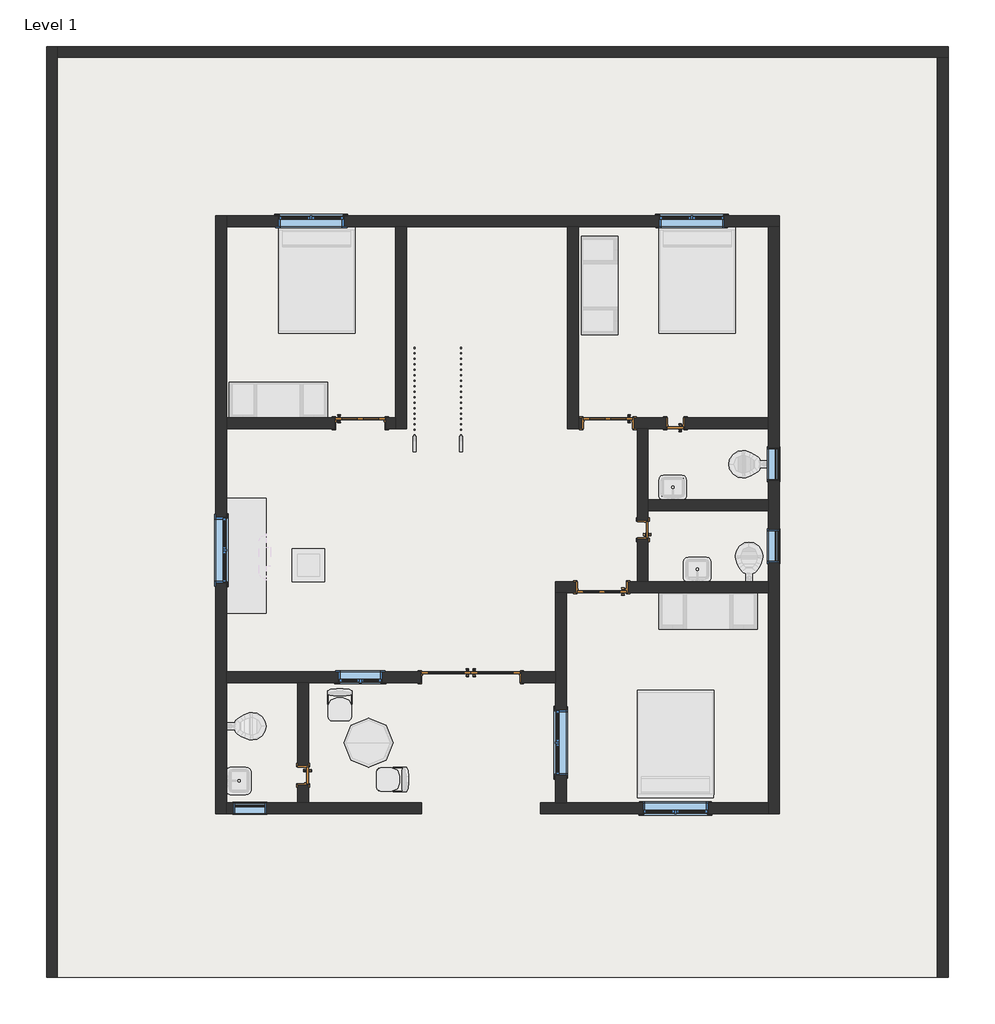
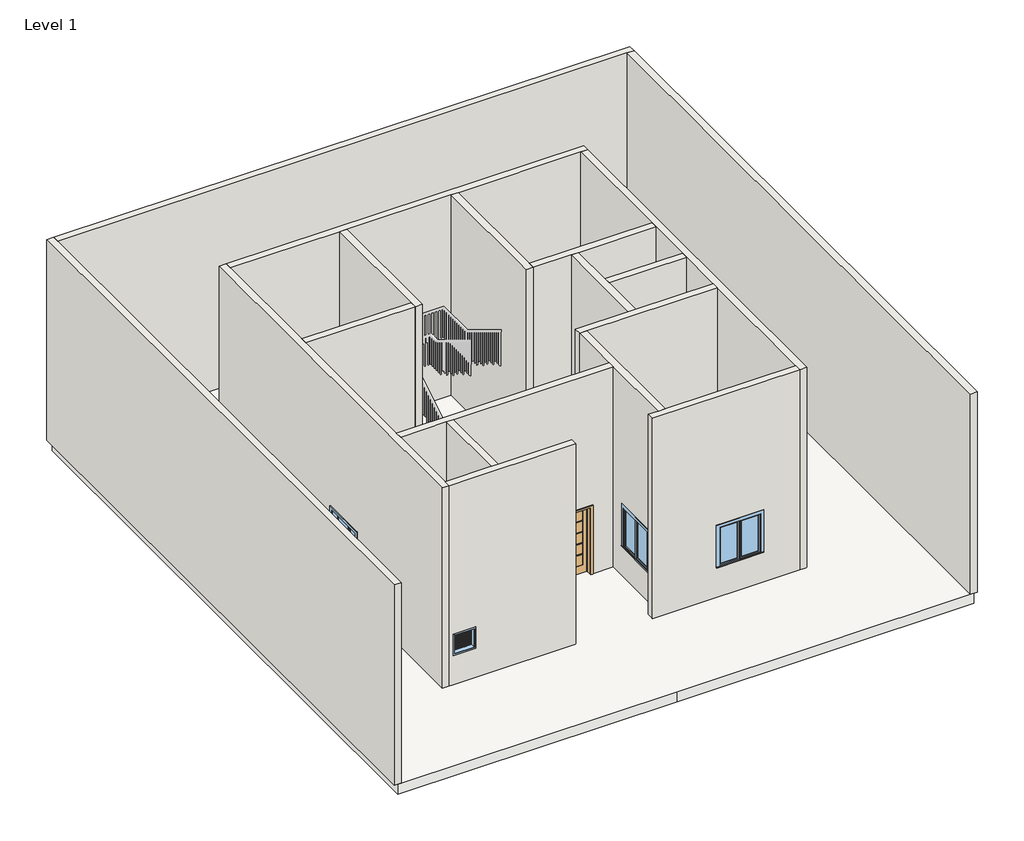
# One storey, part 1 of 3: 18 walls, 9 windows, 7 doors, 1 slab.
"""IFC4 building model written with IfcOpenShell, lengths in millimetres."""

from ifc_helpers import new_model, si_unit, frame, origin, origin_with_axes, place, context, project, spatial, polyline, outline, extrude, faceted_brep, transform, mapped, element, save
from components import door_48c357d2, door_5dfbd760, door_c2afa946, door_21b72c96, door_b2d2822a, window_bb17773d, window_0862ab64, window_0038ecf3, window_75debfae

model = new_model("IFC4")

# Units and contexts
model_context = context("Model", 3, world=origin())
ifc_project = project(units=[si_unit("LENGTHUNIT", "METRE", prefix="MILLI")], contexts=[model_context])

# Site, building, storey
site = spatial("IfcSite", under=ifc_project)
building = spatial("IfcBuilding", under=site)
storey = spatial("IfcBuildingStorey", under=building, Name="Level 1", Elevation=0.0)

# Doors
placement = place(None, origin())
door_shape = door_48c357d2(model_context)
element("IfcDoor", 1, ObjectType="Door-Interior-Double-Full Glass-Wood : 72\" x 80\"", at=placement, inside=storey, context=model_context, shape_type="MappedRepresentation", body=[
    mapped(door_shape, transform((-7146.8868169, 4286.8240268, 0.0), x_axis=(1.0, 0.0, 0.0), y_axis=(0.0, 1.0, 0.0), z_axis=(0.0, 0.0, 1.0))),
])
door_2_shape = door_5dfbd760(model_context)
element("IfcDoor", 2, ObjectType="Door-Interior-Single-6_Panel-Wood : 36\" x 80\"", at=placement, inside=storey, context=model_context, shape_type="MappedRepresentation", body=[
    mapped(door_2_shape, transform((-9204.2868169, 9011.2240268, 0.0), x_axis=(1.0, 0.0, 0.0), y_axis=(0.0, 1.0, 0.0), z_axis=(0.0, 0.0, 1.0))),
])
element("IfcDoor", 3, ObjectType="Door-Interior-Single-6_Panel-Wood : 36\" x 80\"", at=placement, inside=storey, context=model_context, shape_type="MappedRepresentation", body=[
    mapped(door_2_shape, transform((-4708.4868169, 5956.8740268, 0.0), x_axis=(-1.0, 0.0, 0.0), y_axis=(0.0, -1.0, 0.0), z_axis=(0.0, 0.0, 1.0))),
])
door_3_shape = door_c2afa946(model_context)
element("IfcDoor", 4, ObjectType="Door-Interior-Single-6_Panel-Wood : 36\" x 80\"", at=placement, inside=storey, context=model_context, shape_type="MappedRepresentation", body=[
    mapped(door_3_shape, transform((-4594.1868169, 9011.2240268, 0.0), x_axis=(-1.0, 0.0, 0.0), y_axis=(0.0, -1.0, 0.0), z_axis=(0.0, 0.0, 1.0))),
])
door_4_shape = door_21b72c96(model_context)
element("IfcDoor", 5, ObjectType="Door-Interior-Single-Flush_Panel-Wood : 12\" x 80\"", at=placement, inside=storey, context=model_context, shape_type="MappedRepresentation", body=[
    mapped(door_4_shape, transform((-3943.3118169, 7026.8490268, 0.0), x_axis=(0.0, 1.0, 0.0), y_axis=(-1.0, 0.0, 0.0), z_axis=(0.0, 0.0, 1.0))),
])
door_5_shape = door_b2d2822a(model_context)
element("IfcDoor", 6, ObjectType="Door-Interior-Single-Flush_Panel-Wood : 12\" x 80\"", at=placement, inside=storey, context=model_context, shape_type="MappedRepresentation", body=[
    mapped(door_5_shape, transform((-3336.8868169, 9004.8740268, 0.0), x_axis=(-1.0, 0.0, 0.0), y_axis=(0.0, -1.0, 0.0), z_axis=(0.0, 0.0, 1.0))),
])
element("IfcDoor", 7, ObjectType="Door-Interior-Single-Flush_Panel-Wood : 12\" x 80\"", at=placement, inside=storey, context=model_context, shape_type="MappedRepresentation", body=[
    mapped(door_5_shape, transform((-10267.9118169, 2454.8490268, 0.0), x_axis=(0.0, -1.0, 0.0), y_axis=(1.0, 0.0, 0.0), z_axis=(0.0, 0.0, 1.0))),
])

# Slab
element("IfcSlab", 8, ObjectType="Generic - 12\"", at=placement, inside=storey, context=model_context, shape_type="SweptSolid", body=[
    extrude(outline(polyline([(-14944.6868169, 15916.8490268), (1641.5131831, 15916.8490268), (1641.5131831, -1304.3509732), (-6893.7351469, -1304.3509732), (-14944.6868169, -1304.3509732), (-14944.6868169, 15916.8490268)])), frame((0.0, 0.0, -304.8), z_axis=(0.0, 0.0, 1.0), x_axis=(1.0, 0.0, 0.0)), (0.0, 0.0, 1.0), 304.8),
])

# Walls
element("IfcWall", 9, ObjectType="Generic - 8\"", at=placement, inside=storey, context=model_context, shape_type="Brep", body=[
    faceted_brep([(-11693.4868169, 12665.6490268, 0.0), (-8543.8868169, 12665.6490268, 0.0), (-8340.6868169, 12665.6490268, 0.0), (-5343.4868169, 12665.6490268, 0.0), (-5140.2868169, 12665.6490268, 0.0), (-1609.6868169, 12665.6490268, 0.0), (-1406.4868169, 12665.6490268, 0.0), (-1406.4868169, 12665.6490268, 6096.0), (-1609.6868169, 12665.6490268, 6096.0), (-5140.2868169, 12665.6490268, 6096.0), (-5343.4868169, 12665.6490268, 6096.0), (-8340.6868169, 12665.6490268, 6096.0), (-8543.8868169, 12665.6490268, 6096.0), (-11693.4868169, 12665.6490268, 6096.0), (-2422.4868169, 12665.6490268, 2133.6), (-2422.4868169, 12665.6490268, 914.4), (-3641.6868169, 12665.6490268, 914.4), (-3641.6868169, 12665.6490268, 2133.6), (-9509.0868169, 12665.6490268, 2133.6), (-9509.0868169, 12665.6490268, 914.4), (-10728.2868169, 12665.6490268, 914.4), (-10728.2868169, 12665.6490268, 2133.6), (-11693.4868169, 12868.8490268, 0.0), (-11693.4868169, 12868.8490268, 6096.0), (-1406.4868169, 12868.8490268, 6096.0), (-1406.4868169, 12868.8490268, 0.0), (-2422.4868169, 12868.8490268, 2133.6), (-3641.6868169, 12868.8490268, 2133.6), (-3641.6868169, 12868.8490268, 914.4), (-2422.4868169, 12868.8490268, 914.4), (-9509.0868169, 12868.8490268, 2133.6), (-10728.2868169, 12868.8490268, 2133.6), (-10728.2868169, 12868.8490268, 914.4), (-9509.0868169, 12868.8490268, 914.4)], [[[0, 1, 2, 3, 4, 5, 6, 7, 8, 9, 10, 11, 12, 13], [14, 15, 16, 17], [18, 19, 20, 21]], [[22, 23, 24, 25], [26, 27, 28, 29], [30, 31, 32, 33]], [[6, 5, 4, 3, 2, 1, 0, 22, 25]], [[13, 12, 11, 10, 9, 8, 7, 24, 23]], [[7, 6, 25, 24]], [[0, 13, 23, 22]], [[15, 14, 26, 29]], [[16, 15, 29, 28]], [[17, 16, 28, 27]], [[14, 17, 27, 26]], [[19, 18, 30, 33]], [[20, 19, 33, 32]], [[21, 20, 32, 31]], [[18, 21, 31, 30]]]),
])
element("IfcWall", 10, ObjectType="Generic - 8\"", at=placement, inside=storey, context=model_context, shape_type="Brep", body=[
    faceted_brep([(-1609.6868169, 12665.6490268, 0.0), (-1609.6868169, 9109.6490268, 0.0), (-1609.6868169, 8906.4490268, 0.0), (-1609.6868169, 7585.6490268, 0.0), (-1609.6868169, 7382.4490268, 0.0), (-1609.6868169, 6061.6490268, 0.0), (-1609.6868169, 5858.4490268, 0.0), (-1609.6868169, 1946.8490268, 0.0), (-1609.6868169, 1743.6490268, 0.0), (-1609.6868169, 1743.6490268, 6096.0), (-1609.6868169, 1946.8490268, 6096.0), (-1609.6868169, 5858.4490268, 6096.0), (-1609.6868169, 6061.6490268, 6096.0), (-1609.6868169, 7382.4490268, 6096.0), (-1609.6868169, 7585.6490268, 6096.0), (-1609.6868169, 8906.4490268, 6096.0), (-1609.6868169, 9109.6490268, 6096.0), (-1609.6868169, 12665.6490268, 6096.0), (-1609.6868169, 6417.2490268, 1524.0), (-1609.6868169, 6417.2490268, 914.4), (-1609.6868169, 7026.8490268, 914.4), (-1609.6868169, 7026.8490268, 1524.0), (-1609.6868169, 7941.2490268, 1524.0), (-1609.6868169, 7941.2490268, 914.4), (-1609.6868169, 8550.8490268, 914.4), (-1609.6868169, 8550.8490268, 1524.0), (-1406.4868169, 12665.6490268, 0.0), (-1406.4868169, 12665.6490268, 6096.0), (-1406.4868169, 1743.6490268, 6096.0), (-1406.4868169, 1743.6490268, 0.0), (-1406.4868169, 6417.2490268, 1524.0), (-1406.4868169, 7026.8490268, 1524.0), (-1406.4868169, 7026.8490268, 914.4), (-1406.4868169, 6417.2490268, 914.4), (-1406.4868169, 7941.2490268, 1524.0), (-1406.4868169, 8550.8490268, 1524.0), (-1406.4868169, 8550.8490268, 914.4), (-1406.4868169, 7941.2490268, 914.4)], [[[0, 1, 2, 3, 4, 5, 6, 7, 8, 9, 10, 11, 12, 13, 14, 15, 16, 17], [18, 19, 20, 21], [22, 23, 24, 25]], [[26, 27, 28, 29], [30, 31, 32, 33], [34, 35, 36, 37]], [[8, 7, 6, 5, 4, 3, 2, 1, 0, 26, 29]], [[17, 16, 15, 14, 13, 12, 11, 10, 9, 28, 27]], [[0, 17, 27, 26]], [[9, 8, 29, 28]], [[19, 18, 30, 33]], [[20, 19, 33, 32]], [[21, 20, 32, 31]], [[18, 21, 31, 30]], [[23, 22, 34, 37]], [[24, 23, 37, 36]], [[25, 24, 36, 35]], [[22, 25, 35, 34]]]),
])
element("IfcWall", 11, ObjectType="Generic - 8\"", at=placement, inside=storey, context=model_context, shape_type="Brep", body=[
    faceted_brep([(-1609.6868169, 1946.8490268, 0.0), (-5368.8868169, 1946.8490268, 0.0), (-5572.0868169, 1946.8490268, 0.0), (-5851.4868169, 1946.8490268, 0.0), (-5851.4868169, 1946.8490268, 6096.0), (-5572.0868169, 1946.8490268, 6096.0), (-5368.8868169, 1946.8490268, 6096.0), (-1609.6868169, 1946.8490268, 6096.0), (-3946.4868169, 1946.8490268, 2133.6), (-3946.4868169, 1946.8490268, 914.4), (-2727.2868169, 1946.8490268, 914.4), (-2727.2868169, 1946.8490268, 2133.6), (-1609.6868169, 1743.6490268, 0.0), (-1609.6868169, 1743.6490268, 6096.0), (-5851.4868169, 1743.6490268, 6096.0), (-5851.4868169, 1743.6490268, 0.0), (-3946.4868169, 1743.6490268, 2133.6), (-2727.2868169, 1743.6490268, 2133.6), (-2727.2868169, 1743.6490268, 914.4), (-3946.4868169, 1743.6490268, 914.4)], [[[0, 1, 2, 3, 4, 5, 6, 7], [8, 9, 10, 11]], [[12, 13, 14, 15], [16, 17, 18, 19]], [[3, 2, 1, 0, 12, 15]], [[4, 3, 15, 14]], [[7, 6, 5, 4, 14, 13]], [[0, 7, 13, 12]], [[9, 8, 16, 19]], [[10, 9, 19, 18]], [[11, 10, 18, 17]], [[8, 11, 17, 16]]]),
])
element("IfcWall", 12, ObjectType="Generic - 8\"", at=placement, inside=storey, context=model_context, shape_type="Brep", body=[
    faceted_brep([(-11693.4868169, 1743.6490268, 0.0), (-11693.4868169, 1946.8490268, 0.0), (-11693.4868169, 4182.0490268, 0.0), (-11693.4868169, 4385.2490268, 0.0), (-11693.4868169, 8906.4490268, 0.0), (-11693.4868169, 9109.6490268, 0.0), (-11693.4868169, 12665.6490268, 0.0), (-11693.4868169, 12868.8490268, 0.0), (-11693.4868169, 12868.8490268, 6096.0), (-11693.4868169, 12665.6490268, 6096.0), (-11693.4868169, 9109.6490268, 6096.0), (-11693.4868169, 8906.4490268, 6096.0), (-11693.4868169, 4385.2490268, 6096.0), (-11693.4868169, 4182.0490268, 6096.0), (-11693.4868169, 1946.8490268, 6096.0), (-11693.4868169, 1743.6490268, 6096.0), (-11693.4868169, 6036.2490268, 2133.6), (-11693.4868169, 7255.4490268, 2133.6), (-11693.4868169, 7255.4490268, 914.4), (-11693.4868169, 6036.2490268, 914.4), (-11896.6868169, 1743.6490268, 0.0), (-11896.6868169, 1743.6490268, 6096.0), (-11896.6868169, 12868.8490268, 6096.0), (-11896.6868169, 12868.8490268, 0.0), (-11896.6868169, 6036.2490268, 2133.6), (-11896.6868169, 6036.2490268, 914.4), (-11896.6868169, 7255.4490268, 914.4), (-11896.6868169, 7255.4490268, 2133.6)], [[[0, 1, 2, 3, 4, 5, 6, 7, 8, 9, 10, 11, 12, 13, 14, 15], [16, 17, 18, 19]], [[20, 21, 22, 23], [24, 25, 26, 27]], [[7, 6, 5, 4, 3, 2, 1, 0, 20, 23]], [[15, 14, 13, 12, 11, 10, 9, 8, 22, 21]], [[8, 7, 23, 22]], [[0, 15, 21, 20]], [[25, 24, 16, 19]], [[26, 25, 19, 18]], [[27, 26, 18, 17]], [[24, 27, 17, 16]]]),
])
element("IfcWall", 13, ObjectType="Generic - 8\"", at=placement, inside=storey, context=model_context, shape_type="Brep", body=[
    faceted_brep([(-8340.6868169, 8906.4490268, 0.0), (-8340.6868169, 12665.6490268, 0.0), (-8340.6868169, 12665.6490268, 6096.0), (-8340.6868169, 8906.4490268, 6096.0), (-8543.8868169, 8906.4490268, 0.0), (-8543.8868169, 8906.4490268, 6096.0), (-8543.8868169, 9109.6490268, 6096.0), (-8543.8868169, 12665.6490268, 6096.0), (-8543.8868169, 12665.6490268, 0.0), (-8543.8868169, 9109.6490268, 0.0)], [[[0, 1, 2, 3]], [[4, 5, 6, 7, 8, 9]], [[1, 0, 4, 9, 8]], [[3, 2, 7, 6, 5]], [[2, 1, 8, 7]], [[0, 3, 5, 4]]]),
])
element("IfcWall", 14, ObjectType="Generic - 8\"", at=placement, inside=storey, context=model_context, shape_type="Brep", body=[
    faceted_brep([(-5140.2868169, 8906.4490268, 0.0), (-5140.2868169, 9109.6490268, 0.0), (-5140.2868169, 12665.6490268, 0.0), (-5140.2868169, 12665.6490268, 6096.0), (-5140.2868169, 9109.6490268, 6096.0), (-5140.2868169, 8906.4490268, 6096.0), (-5343.4868169, 8906.4490268, 0.0), (-5343.4868169, 8906.4490268, 6096.0), (-5343.4868169, 12665.6490268, 6096.0), (-5343.4868169, 12665.6490268, 0.0)], [[[0, 1, 2, 3, 4, 5]], [[6, 7, 8, 9]], [[2, 1, 0, 6, 9]], [[5, 4, 3, 8, 7]], [[3, 2, 9, 8]], [[0, 5, 7, 6]]]),
])
element("IfcWall", 15, ObjectType="Generic - 8\"", at=placement, inside=storey, context=model_context, shape_type="Brep", body=[
    faceted_brep([(-1609.6868169, 8906.4490268, 6096.0), (-3844.8868169, 8906.4490268, 6096.0), (-4048.0868169, 8906.4490268, 6096.0), (-5140.2868169, 8906.4490268, 6096.0), (-5140.2868169, 8906.4490268, 0.0), (-5076.7868169, 8906.4490268, 0.0), (-5076.7868169, 8906.4490268, 2057.4), (-4111.5868169, 8906.4490268, 2057.4), (-4111.5868169, 8906.4490268, 0.0), (-4048.0868169, 8906.4490268, 0.0), (-3844.8868169, 8906.4490268, 0.0), (-3514.6868169, 8906.4490268, 0.0), (-3514.6868169, 8906.4490268, 2057.4), (-3159.0868169, 8906.4490268, 2057.4), (-3159.0868169, 8906.4490268, 0.0), (-1609.6868169, 8906.4490268, 0.0), (-5140.2868169, 9109.6490268, 6096.0), (-1609.6868169, 9109.6490268, 6096.0), (-1609.6868169, 9109.6490268, 0.0), (-3159.0868169, 9109.6490268, 0.0), (-3159.0868169, 9109.6490268, 2057.4), (-3514.6868169, 9109.6490268, 2057.4), (-3514.6868169, 9109.6490268, 0.0), (-4111.5868169, 9109.6490268, 0.0), (-4111.5868169, 9109.6490268, 2057.4), (-5076.7868169, 9109.6490268, 2057.4), (-5076.7868169, 9109.6490268, 0.0), (-5140.2868169, 9109.6490268, 0.0)], [[[0, 1, 2, 3, 4, 5, 6, 7, 8, 9, 10, 11, 12, 13, 14, 15]], [[16, 17, 18, 19, 20, 21, 22, 23, 24, 25, 26, 27]], [[4, 27, 26, 5]], [[18, 15, 14, 19]], [[8, 23, 22, 11, 10, 9]], [[3, 2, 1, 0, 17, 16]], [[4, 3, 16, 27]], [[0, 15, 18, 17]], [[25, 6, 5, 26]], [[6, 25, 24, 7]], [[7, 24, 23, 8]], [[21, 12, 11, 22]], [[12, 21, 20, 13]], [[13, 20, 19, 14]]]),
])
element("IfcWall", 16, ObjectType="Generic - 8\"", at=placement, inside=storey, context=model_context, shape_type="SweptSolid", body=[
    extrude(outline(polyline([(-1609.6868169, 7382.4490268), (-3844.8868169, 7382.4490268), (-3844.8868169, 7585.6490268), (-1609.6868169, 7585.6490268), (-1609.6868169, 7382.4490268)])), origin_with_axes(), (0.0, 0.0, 1.0), 6096.0),
])
element("IfcWall", 17, ObjectType="Generic - 8\"", at=placement, inside=storey, context=model_context, shape_type="Brep", body=[
    faceted_brep([(-1609.6868169, 5858.4490268, 6096.0), (-5368.8868169, 5858.4490268, 6096.0), (-5572.0868169, 5858.4490268, 6096.0), (-5572.0868169, 5858.4490268, 0.0), (-5368.8868169, 5858.4490268, 0.0), (-5191.0868169, 5858.4490268, 0.0), (-5191.0868169, 5858.4490268, 2057.4), (-4225.8868169, 5858.4490268, 2057.4), (-4225.8868169, 5858.4490268, 0.0), (-1609.6868169, 5858.4490268, 0.0), (-5572.0868169, 6061.6490268, 6096.0), (-4048.0868169, 6061.6490268, 6096.0), (-3844.8868169, 6061.6490268, 6096.0), (-1609.6868169, 6061.6490268, 6096.0), (-1609.6868169, 6061.6490268, 0.0), (-3844.8868169, 6061.6490268, 0.0), (-4048.0868169, 6061.6490268, 0.0), (-4225.8868169, 6061.6490268, 0.0), (-4225.8868169, 6061.6490268, 2057.4), (-5191.0868169, 6061.6490268, 2057.4), (-5191.0868169, 6061.6490268, 0.0), (-5572.0868169, 6061.6490268, 0.0)], [[[0, 1, 2, 3, 4, 5, 6, 7, 8, 9]], [[10, 11, 12, 13, 14, 15, 16, 17, 18, 19, 20, 21]], [[14, 9, 8, 17, 16, 15]], [[3, 21, 20, 5, 4]], [[2, 1, 0, 13, 12, 11, 10]], [[0, 9, 14, 13]], [[3, 2, 10, 21]], [[19, 6, 5, 20]], [[6, 19, 18, 7]], [[7, 18, 17, 8]]]),
])
element("IfcWall", 18, ObjectType="Generic - 8\"", at=placement, inside=storey, context=model_context, shape_type="Brep", body=[
    faceted_brep([(-4048.0868169, 6061.6490268, 6096.0), (-4048.0868169, 8906.4490268, 6096.0), (-4048.0868169, 8906.4490268, 0.0), (-4048.0868169, 7204.6490268, 0.0), (-4048.0868169, 7204.6490268, 2057.4), (-4048.0868169, 6849.0490268, 2057.4), (-4048.0868169, 6849.0490268, 0.0), (-4048.0868169, 6061.6490268, 0.0), (-3844.8868169, 8906.4490268, 6096.0), (-3844.8868169, 7585.6490268, 6096.0), (-3844.8868169, 7382.4490268, 6096.0), (-3844.8868169, 6061.6490268, 6096.0), (-3844.8868169, 6061.6490268, 0.0), (-3844.8868169, 6849.0490268, 0.0), (-3844.8868169, 6849.0490268, 2057.4), (-3844.8868169, 7204.6490268, 2057.4), (-3844.8868169, 7204.6490268, 0.0), (-3844.8868169, 7382.4490268, 0.0), (-3844.8868169, 7585.6490268, 0.0), (-3844.8868169, 8906.4490268, 0.0)], [[[0, 1, 2, 3, 4, 5, 6, 7]], [[8, 9, 10, 11, 12, 13, 14, 15, 16, 17, 18, 19]], [[2, 19, 18, 17, 16, 3]], [[12, 7, 6, 13]], [[1, 0, 11, 10, 9, 8]], [[2, 1, 8, 19]], [[0, 7, 12, 11]], [[15, 4, 3, 16]], [[4, 15, 14, 5]], [[5, 14, 13, 6]]]),
])
element("IfcWall", 19, ObjectType="Generic - 8\"", at=placement, inside=storey, context=model_context, shape_type="Brep", body=[
    faceted_brep([(-5572.0868169, 5858.4490268, 0.0), (-5572.0868169, 4385.2490268, 0.0), (-5572.0868169, 4182.0490268, 0.0), (-5572.0868169, 1946.8490268, 0.0), (-5572.0868169, 1946.8490268, 6096.0), (-5572.0868169, 4182.0490268, 6096.0), (-5572.0868169, 4385.2490268, 6096.0), (-5572.0868169, 5858.4490268, 6096.0), (-5572.0868169, 3674.0490268, 2133.6), (-5572.0868169, 2454.8490268, 2133.6), (-5572.0868169, 2454.8490268, 914.4), (-5572.0868169, 3674.0490268, 914.4), (-5368.8868169, 5858.4490268, 0.0), (-5368.8868169, 5858.4490268, 6096.0), (-5368.8868169, 1946.8490268, 6096.0), (-5368.8868169, 1946.8490268, 0.0), (-5368.8868169, 3674.0490268, 2133.6), (-5368.8868169, 3674.0490268, 914.4), (-5368.8868169, 2454.8490268, 914.4), (-5368.8868169, 2454.8490268, 2133.6)], [[[0, 1, 2, 3, 4, 5, 6, 7], [8, 9, 10, 11]], [[12, 13, 14, 15], [16, 17, 18, 19]], [[3, 2, 1, 0, 12, 15]], [[7, 6, 5, 4, 14, 13]], [[4, 3, 15, 14]], [[0, 7, 13, 12]], [[17, 16, 8, 11]], [[18, 17, 11, 10]], [[19, 18, 10, 9]], [[16, 19, 9, 8]]]),
])
element("IfcWall", 20, ObjectType="Generic - 8\"", at=placement, inside=storey, context=model_context, shape_type="Brep", body=[
    faceted_brep([(-11693.4868169, 4385.2490268, 6096.0), (-5572.0868169, 4385.2490268, 6096.0), (-5572.0868169, 4385.2490268, 0.0), (-6207.0868169, 4385.2490268, 0.0), (-6207.0868169, 4385.2490268, 2057.4), (-8086.6868169, 4385.2490268, 2057.4), (-8086.6868169, 4385.2490268, 0.0), (-11693.4868169, 4385.2490268, 0.0), (-9610.6868169, 4385.2490268, 2133.6), (-9610.6868169, 4385.2490268, 914.4), (-8797.8868169, 4385.2490268, 914.4), (-8797.8868169, 4385.2490268, 2133.6), (-5572.0868169, 4182.0490268, 6096.0), (-10169.4868169, 4182.0490268, 6096.0), (-10372.6868169, 4182.0490268, 6096.0), (-11693.4868169, 4182.0490268, 6096.0), (-11693.4868169, 4182.0490268, 0.0), (-10372.6868169, 4182.0490268, 0.0), (-10169.4868169, 4182.0490268, 0.0), (-8086.6868169, 4182.0490268, 0.0), (-8086.6868169, 4182.0490268, 2057.4), (-6207.0868169, 4182.0490268, 2057.4), (-6207.0868169, 4182.0490268, 0.0), (-5572.0868169, 4182.0490268, 0.0), (-9610.6868169, 4182.0490268, 2133.6), (-8797.8868169, 4182.0490268, 2133.6), (-8797.8868169, 4182.0490268, 914.4), (-9610.6868169, 4182.0490268, 914.4)], [[[0, 1, 2, 3, 4, 5, 6, 7], [8, 9, 10, 11]], [[12, 13, 14, 15, 16, 17, 18, 19, 20, 21, 22, 23], [24, 25, 26, 27]], [[16, 7, 6, 19, 18, 17]], [[2, 23, 22, 3]], [[1, 0, 15, 14, 13, 12]], [[0, 7, 16, 15]], [[2, 1, 12, 23]], [[21, 4, 3, 22]], [[4, 21, 20, 5]], [[5, 20, 19, 6]], [[9, 8, 24, 27]], [[10, 9, 27, 26]], [[11, 10, 26, 25]], [[8, 11, 25, 24]]]),
])
element("IfcWall", 21, ObjectType="Generic - 8\"", at=placement, inside=storey, context=model_context, shape_type="SweptSolid", body=[
    extrude(outline(polyline([(1946.8490268, 6096.0), (4182.0490268, 6096.0), (4182.0490268, 0.0), (2632.6490268, 0.0), (2632.6490268, 2057.4), (2277.0490268, 2057.4), (2277.0490268, 0.0), (1946.8490268, 0.0), (1946.8490268, 6096.0)])), frame((-10372.6868169, 0.0, 0.0), z_axis=(1.0, 0.0, 0.0), x_axis=(0.0, 1.0, 0.0)), (0.0, 0.0, 1.0), 203.2),
])
element("IfcWall", 22, ObjectType="Generic - 8\"", at=placement, inside=storey, context=model_context, shape_type="SweptSolid", body=[
    extrude(outline(polyline([(6096.0, -8543.8868169), (6096.0, -11693.4868169), (0.0, -11693.4868169), (0.0, -9686.8868169), (2057.4, -9686.8868169), (2057.4, -8721.6868169), (0.0, -8721.6868169), (0.0, -8543.8868169), (6096.0, -8543.8868169)])), frame((0.0, 8906.4490268, 0.0), z_axis=(0.0, 1.0, 0.0), x_axis=(0.0, 0.0, 1.0)), (0.0, 0.0, 1.0), 203.2),
])
element("IfcWall", 23, ObjectType="Generic - 8\"", at=placement, inside=storey, context=model_context, shape_type="Brep", body=[
    faceted_brep([(-8061.2868169, 1946.8490268, 0.0), (-10169.4868169, 1946.8490268, 0.0), (-10372.6868169, 1946.8490268, 0.0), (-11693.4868169, 1946.8490268, 0.0), (-11693.4868169, 1946.8490268, 6096.0), (-10372.6868169, 1946.8490268, 6096.0), (-10169.4868169, 1946.8490268, 6096.0), (-8061.2868169, 1946.8490268, 6096.0), (-11566.4868169, 1946.8490268, 1524.0), (-11566.4868169, 1946.8490268, 914.4), (-10956.8868169, 1946.8490268, 914.4), (-10956.8868169, 1946.8490268, 1524.0), (-8061.2868169, 1743.6490268, 0.0), (-8061.2868169, 1743.6490268, 6096.0), (-11693.4868169, 1743.6490268, 6096.0), (-11693.4868169, 1743.6490268, 0.0), (-11566.4868169, 1743.6490268, 1524.0), (-10956.8868169, 1743.6490268, 1524.0), (-10956.8868169, 1743.6490268, 914.4), (-11566.4868169, 1743.6490268, 914.4)], [[[0, 1, 2, 3, 4, 5, 6, 7], [8, 9, 10, 11]], [[12, 13, 14, 15], [16, 17, 18, 19]], [[3, 2, 1, 0, 12, 15]], [[7, 6, 5, 4, 14, 13]], [[0, 7, 13, 12]], [[4, 3, 15, 14]], [[8, 11, 17, 16]], [[11, 10, 18, 17]], [[10, 9, 19, 18]], [[9, 8, 16, 19]]]),
])
element("IfcWall", 24, ObjectType="Generic - 8\"", at=placement, inside=storey, context=model_context, shape_type="Brep", body=[
    faceted_brep([(-14843.0868169, -1304.3509732, 0.0), (-14843.0868169, 15815.2490268, 0.0), (-14843.0868169, 16018.4490268, 0.0), (-14843.0868169, 16018.4490268, 6096.0), (-14843.0868169, 15815.2490268, 6096.0), (-14843.0868169, -1304.3509732, 6096.0), (-15046.2868169, -1304.3509732, 0.0), (-15046.2868169, -1304.3509732, 6096.0), (-15046.2868169, 16018.4490268, 6096.0), (-15046.2868169, 16018.4490268, 0.0)], [[[0, 1, 2, 3, 4, 5]], [[6, 7, 8, 9]], [[2, 1, 0, 6, 9]], [[5, 4, 3, 8, 7]], [[0, 5, 7, 6]], [[3, 2, 9, 8]]]),
])
element("IfcWall", 25, ObjectType="Generic - 8\"", at=placement, inside=storey, context=model_context, shape_type="Brep", body=[
    faceted_brep([(-14843.0868169, 15815.2490268, 0.0), (1539.9131831, 15815.2490268, 0.0), (1743.1131831, 15815.2490268, 0.0), (1743.1131831, 15815.2490268, 6096.0), (1539.9131831, 15815.2490268, 6096.0), (-14843.0868169, 15815.2490268, 6096.0), (-14843.0868169, 16018.4490268, 0.0), (-14843.0868169, 16018.4490268, 6096.0), (1743.1131831, 16018.4490268, 6096.0), (1743.1131831, 16018.4490268, 0.0)], [[[0, 1, 2, 3, 4, 5]], [[6, 7, 8, 9]], [[2, 1, 0, 6, 9]], [[5, 4, 3, 8, 7]], [[0, 5, 7, 6]], [[3, 2, 9, 8]]]),
])
element("IfcWall", 26, ObjectType="Generic - 8\"", at=placement, inside=storey, context=model_context, shape_type="SweptSolid", body=[
    extrude(outline(polyline([(1539.9131831, -1304.3509732), (1539.9131831, 15815.2490268), (1743.1131831, 15815.2490268), (1743.1131831, -1304.3509732), (1539.9131831, -1304.3509732)])), origin_with_axes(), (0.0, 0.0, 1.0), 6096.0),
])

# Windows
window_shape = window_bb17773d(model_context)
element("IfcWindow", 27, ObjectType="Casement Dbl with Trim : 32\" x 48\"", at=placement, inside=storey, context=model_context, shape_type="MappedRepresentation", body=[
    mapped(window_shape, transform((-9204.2868169, 4302.6990268, 0.0), x_axis=(-1.0, 0.0, 0.0), y_axis=(0.0, -1.0, 0.0), z_axis=(0.0, 0.0, 1.0))),
])
window_2_shape = window_0862ab64(model_context)
element("IfcWindow", 28, ObjectType="Casement Dbl with Trim : 48\" x 48\"", at=placement, inside=storey, context=model_context, shape_type="MappedRepresentation", body=[
    mapped(window_2_shape, transform((-3336.8868169, 1864.2990268, 0.0), x_axis=(-1.0, 0.0, 0.0), y_axis=(0.0, -1.0, 0.0), z_axis=(0.0, 0.0, 1.0))),
])
element("IfcWindow", 29, ObjectType="Casement Dbl with Trim : 48\" x 48\"", at=placement, inside=storey, context=model_context, shape_type="MappedRepresentation", body=[
    mapped(window_2_shape, transform((-5451.4368169, 3064.4490268, 0.0), x_axis=(0.0, 1.0, 0.0), y_axis=(-1.0, 0.0, 0.0), z_axis=(0.0, 0.0, 1.0))),
])
element("IfcWindow", 30, ObjectType="Casement Dbl with Trim : 48\" x 48\"", at=placement, inside=storey, context=model_context, shape_type="MappedRepresentation", body=[
    mapped(window_2_shape, transform((-3032.0868169, 12748.1990268, 0.0), x_axis=(1.0, 0.0, 0.0), y_axis=(0.0, 1.0, 0.0), z_axis=(0.0, 0.0, 1.0))),
])
element("IfcWindow", 31, ObjectType="Casement Dbl with Trim : 48\" x 48\"", at=placement, inside=storey, context=model_context, shape_type="MappedRepresentation", body=[
    mapped(window_2_shape, transform((-10118.6868169, 12748.1990268, 0.0), x_axis=(1.0, 0.0, 0.0), y_axis=(0.0, 1.0, 0.0), z_axis=(0.0, 0.0, 1.0))),
])
element("IfcWindow", 32, ObjectType="Casement Dbl with Trim : 48\" x 48\"", at=placement, inside=storey, context=model_context, shape_type="MappedRepresentation", body=[
    mapped(window_2_shape, transform((-11814.1368169, 6645.8490268, 0.0), x_axis=(0.0, -1.0, 0.0), y_axis=(1.0, 0.0, 0.0), z_axis=(0.0, 0.0, 1.0))),
])
window_3_shape = window_0038ecf3(model_context)
element("IfcWindow", 33, ObjectType="Louvers with Trim : 24\" x 24\"", at=placement, inside=storey, context=model_context, shape_type="MappedRepresentation", body=[
    mapped(window_3_shape, transform((-1501.7368169, 6722.0490268, 0.0), x_axis=(0.0, -1.0, 0.0), y_axis=(1.0, 0.0, 0.0), z_axis=(0.0, 0.0, 1.0))),
])
element("IfcWindow", 34, ObjectType="Louvers with Trim : 24\" x 24\"", at=placement, inside=storey, context=model_context, shape_type="MappedRepresentation", body=[
    mapped(window_3_shape, transform((-1501.7368169, 8246.0490268, 0.0), x_axis=(0.0, -1.0, 0.0), y_axis=(1.0, 0.0, 0.0), z_axis=(0.0, 0.0, 1.0))),
])
window_4_shape = window_75debfae(model_context)
element("IfcWindow", 35, ObjectType="Louvers with Trim : 24\" x 24\"", at=placement, inside=storey, context=model_context, shape_type="MappedRepresentation", body=[
    mapped(window_4_shape, transform((-11261.6868169, 1851.5990268, 0.0), x_axis=(-1.0, 0.0, 0.0), y_axis=(0.0, -1.0, 0.0), z_axis=(0.0, 0.0, 1.0))),
])

save(model, "model.ifc")

# Revit data of these elements
# Type "Door-Interior-Double-Full Glass-Wood : 72\" x 80\""
#   Type Mark = "8"
#   Assembly Code = "C1020300"
#   Analytic Construction = "French door, wood frame with single glass"
#   Top Rail = 0' - 4 11/16"
#   Thickness = 0' - 1 3/8"
#   Thermal Resistance (R) = 1.0696 (h·ft²·°F)/BTU
#   Swing Angle [instance default] = 90.00°
#   Stiles = 0' - 4 3/4"
#   Rough Width = 6' - 2"
#   Rough Height = 6' - 9"
#   Panel Width = 3' - 0"
#   Height = 6' - 8"
#   Width = 6' - 0"
#   Heat Transfer Coefficient (U) = 0.9350 BTU/(h·ft²·°F)
#   Bottom Rail = 0' - 9 1/8"
#   Show Grill [instance default] = yes
#   Trim Material = Cherry
#   Panel Material = Cherry
#   Frame Material = Cherry
#   Door Handle Material = Aluminum
#   Visual Light Transmittance = 0
#   Solar Heat Gain Coefficient = 0
#   Wall Closure = (empty or 0)
#   Function = (empty or 0)
# Type "Door-Interior-Single-6_Panel-Wood : 36\" x 80\""
#   Type Mark = "9"
#   Assembly Code = "C1020300"
#   Analytic Construction = "Wooden"
#   Top Rail = 0' - 4 11/16"
#   Top Panel = 0' - 11"
#   Thickness = 0' - 1 3/8"
#   Thermal Resistance (R) = 2.5876 (h·ft²·°F)/BTU
#   Swing Angle [instance default] = 90.00°
#   Stiles = 0' - 4 3/4"
#   Rough Width = 3' - 2"
#   Rough Height = 6' - 9"
#   Mullion = 0' - 4 1/2"
#   Lock Rail = 0' - 7 1/2"
#   Intermediate Rail = 0' - 4 1/2"
#   Height = 6' - 8"
#   Width = 3' - 0"
#   Heat Transfer Coefficient (U) = 0.3865 BTU/(h·ft²·°F)
#   Bottom Rail = 0' - 9 1/8"
#   Trim Material = Cherry
#   Panel Material = Cherry
#   Frame Material = Cherry
#   Door Handle Material = Aluminum
#   Visual Light Transmittance = 0
#   Solar Heat Gain Coefficient = 0
#   Wall Closure = (empty or 0)
#   Function = (empty or 0)
# Type "Door-Interior-Single-Flush_Panel-Wood : 12\" x 80\""
#   Type Mark = "10"
#   Assembly Code = "C1020300"
#   Analytic Construction = "Wooden"
#   Thickness = 0' - 1 3/8"
#   Thermal Resistance (R) = 2.5876 (h·ft²·°F)/BTU
#   Swing Angle [instance default] = 90.00°
#   Rough Width = 1' - 2"
#   Rough Height = 6' - 9"
#   Height = 6' - 8"
#   Width = 1' - 0"
#   Heat Transfer Coefficient (U) = 0.3865 BTU/(h·ft²·°F)
#   Trim Material = Cherry
#   Panel Material = Cherry
#   Frame Material = Cherry
#   Door Handle Material = Aluminum
#   Visual Light Transmittance = 0
#   Solar Heat Gain Coefficient = 0
#   Wall Closure = (empty or 0)
#   Function = (empty or 0)
# Type "Generic - 12\""
#   Assembly Code = "B1010"
#   Function = 0
#   Layers, outside or top first: 1' - 0" "Default New Material" (function 1)
# Type "Generic - 8\""
#   Assembly Code = "B2010"
#   Layers, outside or top first: 0' - 8" no material (function 1)
# Type "Casement Dbl with Trim : 32\" x 48\""
#   Type Mark = "19"
#   Construction Type Id = "GSP4R"
#   Assembly Code = "B2020100"
#   Analytic Construction = "1/8 in Pilkington single glazing"
#   Visual Light Transmittance = 0.9
#   Solar Heat Gain Coefficient = 0.78
#   Heat Transfer Coefficient (U) = 0.6496 BTU/(h·ft²·°F)
#   Height = 4' - 0"
#   Default Sill Height = 3' - 0"
#   Trim Projection - Ext. = 0' - 0 1/2"
#   Trim Projection - Int. = 0' - 0 3/4"
#   Trim Width - Exterior = 0' - 3 1/2"
#   Trim Width - Interior = 0' - 3 1/2"
#   Width = 2' - 8"
#   Window Inset = 0' - 0 3/4"
#   Define Thermal Properties by = 1
#   Glass Pane Material = Glass
#   Sash Material = Sash
#   Trim Exterior Material = Trim
#   Trim Interior Material = Trim
#   Wall Closure = (empty or 0)
# Type "Casement Dbl with Trim : 48\" x 48\""
#   Type Mark = "17"
#   Construction Type Id = "GSP4R"
#   Assembly Code = "B2020100"
#   Analytic Construction = "1/8 in Pilkington single glazing"
#   Visual Light Transmittance = 0.9
#   Solar Heat Gain Coefficient = 0.78
#   Heat Transfer Coefficient (U) = 0.6496 BTU/(h·ft²·°F)
#   Height = 4' - 0"
#   Default Sill Height = 3' - 0"
#   Trim Projection - Ext. = 0' - 0 1/2"
#   Trim Projection - Int. = 0' - 0 3/4"
#   Trim Width - Exterior = 0' - 3 1/2"
#   Trim Width - Interior = 0' - 3 1/2"
#   Width = 4' - 0"
#   Window Inset = 0' - 0 3/4"
#   Define Thermal Properties by = 1
#   Glass Pane Material = Glass
#   Sash Material = Sash
#   Trim Exterior Material = Trim
#   Trim Interior Material = Trim
#   Wall Closure = (empty or 0)
# Type "Louvers with Trim : 24\" x 24\""
#   Type Mark = "10"
#   Construction Type Id = "GSP4R"
#   Assembly Code = "B20"
#   Analytic Construction = "1/8 in Pilkington single glazing"
#   Visual Light Transmittance = 0.9
#   Solar Heat Gain Coefficient = 0.78
#   Heat Transfer Coefficient (U) = 0.6496 BTU/(h·ft²·°F)
#   Default Sill Height = 3' - 0"
#   Trim Projection - Ext. = 0' - 0 1/2"
#   Trim Projection - Int. = 0' - 0 1/2"
#   Trim Width - Exterior = 0' - 1 1/2"
#   Trim Width - Interior = 0' - 1 1/2"
#   Width = 2' - 0"
#   Define Thermal Properties by = 1
#   Frame Material = Birch
#   Louver Material = Birch
#   Trim Exterior Material = Birch
#   Trim Interior Material = Birch
#   Wall Closure = (empty or 0)
# Element 1 (IfcDoor, "Door-Interior-Double-Full Glass-Wood : 72\" x 80\"")
#   Swing Angle = 90.00°
#   Show Grill = yes
#   Phase Created = New Construction
#   Materials on its faces: "Cherry", "Aluminum", "Glass"
# Elements 2, 3, 4 (IfcDoor, "Door-Interior-Single-6_Panel-Wood : 36\" x 80\"")
#   Swing Angle = 90.00°
#   Phase Created = New Construction
#   Materials on its faces: "Cherry", "Aluminum"
# Elements 5, 6, 7 (IfcDoor, "Door-Interior-Single-Flush_Panel-Wood : 12\" x 80\"")
#   Swing Angle = 90.00°
#   Phase Created = New Construction
#   Materials on its faces: "Cherry", "Aluminum"
# Element 8 (IfcSlab, "Generic - 12\"")
#   built-in parameter 1001955 = 1.5708 (stored number, unit not read)
#   Height Offset From Level = 0' - 0"
#   Phase Created = New Construction
#   Materials on its faces: "Default New Material"
# Elements 9, 10, 11, 12, 13, 14, 15, 16, 17, 18, 19, 20, 21, 22, 23, 24, 25, 26 (IfcWall, "Generic - 8\"")
#   Top Offset = 0' - 0"
#   Base Offset = 0' - 0"
#   Unconnected Height = 20' - 0"
#   wall height = 20' - 0"
#   Phase Created = New Construction
#   Base Constraint = Level 1
#   Materials on its faces: "Default Wall"
# Element 27 (IfcWindow, "Casement Dbl with Trim : 32\" x 48\"")
#   Mark = "8"
#   Phase Created = New Construction
#   Materials on its faces: "Sash", "Trim", "Glass"
# Element 28 (IfcWindow, "Casement Dbl with Trim : 48\" x 48\"")
#   Mark = "4"
#   Phase Created = New Construction
#   Materials on its faces: "Sash", "Trim", "Glass"
# Element 29 (IfcWindow, "Casement Dbl with Trim : 48\" x 48\"")
#   Mark = "5"
#   Phase Created = New Construction
#   Materials on its faces: "Sash", "Trim", "Glass"
# Element 30 (IfcWindow, "Casement Dbl with Trim : 48\" x 48\"")
#   Mark = "6"
#   Phase Created = New Construction
#   Materials on its faces: "Sash", "Trim", "Glass"
# Element 31 (IfcWindow, "Casement Dbl with Trim : 48\" x 48\"")
#   Mark = "7"
#   Phase Created = New Construction
#   Materials on its faces: "Sash", "Trim", "Glass"
# Element 32 (IfcWindow, "Casement Dbl with Trim : 48\" x 48\"")
#   Mark = "9"
#   Phase Created = New Construction
#   Materials on its faces: "Sash", "Trim", "Glass"
# Element 33 (IfcWindow, "Louvers with Trim : 24\" x 24\"")
#   Mark = "1"
#   Phase Created = New Construction
#   Materials on its faces: "Birch"
# Element 34 (IfcWindow, "Louvers with Trim : 24\" x 24\"")
#   Mark = "2"
#   Phase Created = New Construction
#   Materials on its faces: "Birch"
# Element 35 (IfcWindow, "Louvers with Trim : 24\" x 24\"")
#   Mark = "3"
#   Phase Created = New Construction
#   Materials on its faces: "Birch"
# Materials
#   "Cherry": class "Wood", colour RGB 226 177 128, transparency 0, Description = "Prunus Serotina", Cost = 0
#   "Aluminum": class "Metal", colour RGB 247 247 247, transparency 0, Description = "Aluminum 6061", Cost = 0
#   "Default New Material": class "Generic", colour RGB 120 120 120, transparency 0, Cost = 0
#   "Glass": class "Glass", colour RGB 0 128 192, transparency 0.75, Description = "Soda Lime Glass", Cost = 0
#   "Sash": class "Wood", colour RGB 224 178 126, transparency 0
#   "Trim": class "Wood", colour RGB 224 178 126, transparency 0
#   "Birch": class "Wood", colour RGB 224 178 126, transparency 0, Description = "Betula Alleghaniensis", Cost = 0
#   "Default Wall": colour RGB 128 128 128, transparency 0
